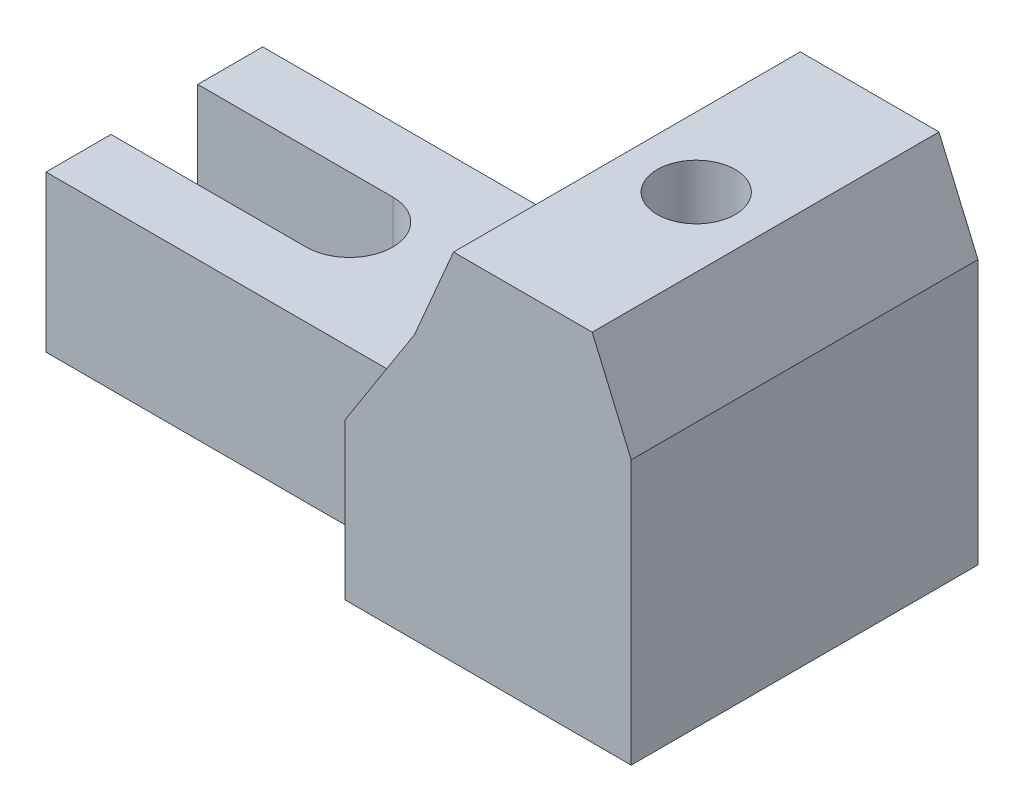
ISO-10303-21;
HEADER;
FILE_DESCRIPTION(('STEP AP214'),'2;1');
FILE_NAME('part.step','',(''),(''),'','','');
FILE_SCHEMA(('AUTOMOTIVE_DESIGN { 1 0 10303 214 1 1 1 1 }'));
ENDSEC;
DATA;
#1=APPLICATION_CONTEXT('core data for automotive mechanical design processes');
#2=APPLICATION_PROTOCOL_DEFINITION('international standard','automotive_design',2000,#1);
#3=PRODUCT_CONTEXT('',#1,'mechanical');
#4=PRODUCT('Part','Part','',(#3));
#5=PRODUCT_RELATED_PRODUCT_CATEGORY('part','',(#4));
#6=PRODUCT_DEFINITION_FORMATION('','',#4);
#7=PRODUCT_DEFINITION_CONTEXT('part definition',#1,'design');
#8=PRODUCT_DEFINITION('design','',#6,#7);
#9=PRODUCT_DEFINITION_SHAPE('','',#8);
#10=(LENGTH_UNIT() NAMED_UNIT(*) SI_UNIT(.MILLI.,.METRE.));
#11=(NAMED_UNIT(*) PLANE_ANGLE_UNIT() SI_UNIT($,.RADIAN.));
#12=(NAMED_UNIT(*) SI_UNIT($,.STERADIAN.) SOLID_ANGLE_UNIT());
#13=UNCERTAINTY_MEASURE_WITH_UNIT(LENGTH_MEASURE(1.E-05),#10,'distance_accuracy_value','');
#14=(GEOMETRIC_REPRESENTATION_CONTEXT(3) GLOBAL_UNCERTAINTY_ASSIGNED_CONTEXT((#13)) GLOBAL_UNIT_ASSIGNED_CONTEXT((#10,
#11,#12)) REPRESENTATION_CONTEXT('',''));
#15=CARTESIAN_POINT('',(0.,0.,0.));
#16=DIRECTION('',(0.,0.,1.));
#17=DIRECTION('',(1.,0.,0.));
#18=AXIS2_PLACEMENT_3D('',#15,#16,#17);
#19=CARTESIAN_POINT('',(0.,0.,80.));
#20=DIRECTION('',(1.,0.,0.));
#21=DIRECTION('',(0.,0.,-1.));
#22=AXIS2_PLACEMENT_3D('',#19,#20,#21);
#23=PLANE('',#22);
#24=DIRECTION('',(0.,-1.,0.));
#25=VECTOR('',#24,1.);
#26=CARTESIAN_POINT('',(0.,36.,15.));
#27=LINE('',#26,#25);
#28=CARTESIAN_POINT('',(0.,36.,15.));
#29=VERTEX_POINT('',#28);
#30=CARTESIAN_POINT('',(0.,0.,15.));
#31=VERTEX_POINT('',#30);
#32=EDGE_CURVE('E177',#29,#31,#27,.T.);
#33=ORIENTED_EDGE('',*,*,#32,.F.);
#34=DIRECTION('',(0.,0.,-1.));
#35=VECTOR('',#34,1.);
#36=CARTESIAN_POINT('',(0.,36.,80.));
#37=LINE('',#36,#35);
#38=CARTESIAN_POINT('',(0.,36.,0.));
#39=VERTEX_POINT('',#38);
#40=EDGE_CURVE('E93',#29,#39,#37,.T.);
#41=ORIENTED_EDGE('',*,*,#40,.T.);
#42=DIRECTION('',(0.,-1.,0.));
#43=VECTOR('',#42,1.);
#44=CARTESIAN_POINT('',(0.,0.,0.));
#45=LINE('',#44,#43);
#46=CARTESIAN_POINT('',(0.,0.,0.));
#47=VERTEX_POINT('',#46);
#48=EDGE_CURVE('E145',#39,#47,#45,.T.);
#49=ORIENTED_EDGE('',*,*,#48,.T.);
#50=DIRECTION('',(0.,0.,-1.));
#51=VECTOR('',#50,1.);
#52=CARTESIAN_POINT('',(0.,0.,80.));
#53=LINE('',#52,#51);
#54=EDGE_CURVE('E52',#31,#47,#53,.T.);
#55=ORIENTED_EDGE('',*,*,#54,.F.);
#56=EDGE_LOOP('',(#33,#41,#49,#55));
#57=FACE_BOUND('',#56,.T.);
#58=ADVANCED_FACE('F44',(#57),#23,.F.);
#59=CARTESIAN_POINT('',(0.,36.,80.));
#60=VERTEX_POINT('',#59);
#61=CARTESIAN_POINT('',(0.,36.,65.));
#62=VERTEX_POINT('',#61);
#63=EDGE_CURVE('E157',#60,#62,#37,.T.);
#64=ORIENTED_EDGE('',*,*,#63,.T.);
#65=DIRECTION('',(0.,-1.,0.));
#66=VECTOR('',#65,1.);
#67=CARTESIAN_POINT('',(0.,36.,65.));
#68=LINE('',#67,#66);
#69=CARTESIAN_POINT('',(0.,0.,65.));
#70=VERTEX_POINT('',#69);
#71=EDGE_CURVE('E186',#62,#70,#68,.T.);
#72=ORIENTED_EDGE('',*,*,#71,.T.);
#73=CARTESIAN_POINT('',(0.,0.,80.));
#74=VERTEX_POINT('',#73);
#75=EDGE_CURVE('E11',#74,#70,#53,.T.);
#76=ORIENTED_EDGE('',*,*,#75,.F.);
#77=DIRECTION('',(0.,-1.,0.));
#78=VECTOR('',#77,1.);
#79=CARTESIAN_POINT('',(0.,0.,80.));
#80=LINE('',#79,#78);
#81=EDGE_CURVE('E149',#60,#74,#80,.T.);
#82=ORIENTED_EDGE('',*,*,#81,.F.);
#83=EDGE_LOOP('',(#64,#72,#76,#82));
#84=FACE_BOUND('',#83,.T.);
#85=ADVANCED_FACE('F50',(#84),#23,.F.);
#86=CARTESIAN_POINT('',(0.,0.,80.));
#87=DIRECTION('',(0.,1.,0.));
#88=DIRECTION('',(0.,0.,1.));
#89=AXIS2_PLACEMENT_3D('',#86,#87,#88);
#90=PLANE('',#89);
#91=DIRECTION('',(1.,0.,0.));
#92=VECTOR('',#91,1.);
#93=CARTESIAN_POINT('',(0.,0.,0.));
#94=LINE('',#93,#92);
#95=CARTESIAN_POINT('',(66.,0.,0.));
#96=VERTEX_POINT('',#95);
#97=EDGE_CURVE('E154',#47,#96,#94,.T.);
#98=ORIENTED_EDGE('',*,*,#97,.T.);
#99=DIRECTION('',(0.,0.,-1.));
#100=VECTOR('',#99,1.);
#101=CARTESIAN_POINT('',(66.,0.,80.));
#102=LINE('',#101,#100);
#103=CARTESIAN_POINT('',(66.,0.,80.));
#104=VERTEX_POINT('',#103);
#105=EDGE_CURVE('E130',#104,#96,#102,.T.);
#106=ORIENTED_EDGE('',*,*,#105,.F.);
#107=DIRECTION('',(1.,0.,0.));
#108=VECTOR('',#107,1.);
#109=CARTESIAN_POINT('',(0.,0.,80.));
#110=LINE('',#109,#108);
#111=EDGE_CURVE('E97',#74,#104,#110,.T.);
#112=ORIENTED_EDGE('',*,*,#111,.F.);
#113=ORIENTED_EDGE('',*,*,#75,.T.);
#114=DIRECTION('',(-1.,0.,0.));
#115=VECTOR('',#114,1.);
#116=CARTESIAN_POINT('',(0.,0.,65.));
#117=LINE('',#116,#115);
#118=CARTESIAN_POINT('',(-84.,0.,65.));
#119=VERTEX_POINT('',#118);
#120=EDGE_CURVE('E58',#70,#119,#117,.T.);
#121=ORIENTED_EDGE('',*,*,#120,.T.);
#122=DIRECTION('',(0.,0.,-1.));
#123=VECTOR('',#122,1.);
#124=CARTESIAN_POINT('',(-84.,0.,65.));
#125=LINE('',#124,#123);
#126=CARTESIAN_POINT('',(-84.,0.,50.));
#127=VERTEX_POINT('',#126);
#128=EDGE_CURVE('E215',#119,#127,#125,.T.);
#129=ORIENTED_EDGE('',*,*,#128,.T.);
#130=DIRECTION('',(1.,0.,0.));
#131=VECTOR('',#130,1.);
#132=CARTESIAN_POINT('',(-39.,0.,50.));
#133=LINE('',#132,#131);
#134=CARTESIAN_POINT('',(-39.,0.,50.));
#135=VERTEX_POINT('',#134);
#136=EDGE_CURVE('E214',#127,#135,#133,.T.);
#137=ORIENTED_EDGE('',*,*,#136,.T.);
#138=CARTESIAN_POINT('',(-39.,0.,40.));
#139=DIRECTION('',(0.,1.,0.));
#140=DIRECTION('',(0.,0.,-1.));
#141=AXIS2_PLACEMENT_3D('',#138,#139,#140);
#142=CIRCLE('',#141,10.);
#143=CARTESIAN_POINT('',(-39.,0.,30.));
#144=VERTEX_POINT('',#143);
#145=EDGE_CURVE('E217',#135,#144,#142,.T.);
#146=ORIENTED_EDGE('',*,*,#145,.T.);
#147=DIRECTION('',(-1.,0.,0.));
#148=VECTOR('',#147,1.);
#149=CARTESIAN_POINT('',(-39.,0.,30.));
#150=LINE('',#149,#148);
#151=CARTESIAN_POINT('',(-84.,0.,30.));
#152=VERTEX_POINT('',#151);
#153=EDGE_CURVE('E222',#144,#152,#150,.T.);
#154=ORIENTED_EDGE('',*,*,#153,.T.);
#155=DIRECTION('',(0.,0.,-1.));
#156=VECTOR('',#155,1.);
#157=CARTESIAN_POINT('',(-84.,0.,15.));
#158=LINE('',#157,#156);
#159=CARTESIAN_POINT('',(-84.,0.,15.));
#160=VERTEX_POINT('',#159);
#161=EDGE_CURVE('E221',#152,#160,#158,.T.);
#162=ORIENTED_EDGE('',*,*,#161,.T.);
#163=DIRECTION('',(1.,0.,0.));
#164=VECTOR('',#163,1.);
#165=CARTESIAN_POINT('',(0.,0.,15.));
#166=LINE('',#165,#164);
#167=EDGE_CURVE('E166',#160,#31,#166,.T.);
#168=ORIENTED_EDGE('',*,*,#167,.T.);
#169=ORIENTED_EDGE('',*,*,#54,.T.);
#170=EDGE_LOOP('',(#98,#106,#112,#113,#121,#129,#137,#146,#154,#162,#168,#169));
#171=FACE_BOUND('',#170,.T.);
#172=ADVANCED_FACE('F164',(#171),#90,.F.);
#173=CARTESIAN_POINT('',(66.,0.,80.));
#174=DIRECTION('',(-1.,0.,0.));
#175=DIRECTION('',(0.,0.,1.));
#176=AXIS2_PLACEMENT_3D('',#173,#174,#175);
#177=PLANE('',#176);
#178=DIRECTION('',(0.,1.,0.));
#179=VECTOR('',#178,1.);
#180=CARTESIAN_POINT('',(66.,0.,0.));
#181=LINE('',#180,#179);
#182=CARTESIAN_POINT('',(66.,61.,0.));
#183=VERTEX_POINT('',#182);
#184=EDGE_CURVE('E124',#96,#183,#181,.T.);
#185=ORIENTED_EDGE('',*,*,#184,.T.);
#186=DIRECTION('',(0.,0.,-1.));
#187=VECTOR('',#186,1.);
#188=CARTESIAN_POINT('',(66.,61.,80.));
#189=LINE('',#188,#187);
#190=CARTESIAN_POINT('',(66.,61.,80.));
#191=VERTEX_POINT('',#190);
#192=EDGE_CURVE('E116',#191,#183,#189,.T.);
#193=ORIENTED_EDGE('',*,*,#192,.F.);
#194=DIRECTION('',(0.,1.,0.));
#195=VECTOR('',#194,1.);
#196=CARTESIAN_POINT('',(66.,0.,80.));
#197=LINE('',#196,#195);
#198=EDGE_CURVE('E110',#104,#191,#197,.T.);
#199=ORIENTED_EDGE('',*,*,#198,.F.);
#200=ORIENTED_EDGE('',*,*,#105,.T.);
#201=EDGE_LOOP('',(#185,#193,#199,#200));
#202=FACE_BOUND('',#201,.T.);
#203=ADVANCED_FACE('F118',(#202),#177,.F.);
#204=CARTESIAN_POINT('',(16.,61.,80.));
#205=DIRECTION('',(0.842271400661511,-0.539053696423367,0.));
#206=DIRECTION('',(0.539053696423367,0.842271400661511,0.));
#207=AXIS2_PLACEMENT_3D('',#204,#205,#206);
#208=PLANE('',#207);
#209=DIRECTION('',(-0.539053696423367,-0.842271400661511,0.));
#210=VECTOR('',#209,1.);
#211=CARTESIAN_POINT('',(16.,61.,0.));
#212=LINE('',#211,#210);
#213=CARTESIAN_POINT('',(16.,61.,0.));
#214=VERTEX_POINT('',#213);
#215=EDGE_CURVE('E151',#214,#39,#212,.T.);
#216=ORIENTED_EDGE('',*,*,#215,.T.);
#217=ORIENTED_EDGE('',*,*,#40,.F.);
#218=DIRECTION('',(0.,0.,1.));
#219=VECTOR('',#218,1.);
#220=CARTESIAN_POINT('',(0.,36.,65.));
#221=LINE('',#220,#219);
#222=EDGE_CURVE('E197',#29,#62,#221,.T.);
#223=ORIENTED_EDGE('',*,*,#222,.T.);
#224=ORIENTED_EDGE('',*,*,#63,.F.);
#225=DIRECTION('',(-0.539053696423367,-0.842271400661511,0.));
#226=VECTOR('',#225,1.);
#227=CARTESIAN_POINT('',(16.,61.,80.));
#228=LINE('',#227,#226);
#229=CARTESIAN_POINT('',(16.,61.,80.));
#230=VERTEX_POINT('',#229);
#231=EDGE_CURVE('E66',#230,#60,#228,.T.);
#232=ORIENTED_EDGE('',*,*,#231,.F.);
#233=DIRECTION('',(0.,0.,-1.));
#234=VECTOR('',#233,1.);
#235=CARTESIAN_POINT('',(16.,61.,80.));
#236=LINE('',#235,#234);
#237=EDGE_CURVE('E126',#230,#214,#236,.T.);
#238=ORIENTED_EDGE('',*,*,#237,.T.);
#239=EDGE_LOOP('',(#216,#217,#223,#224,#232,#238));
#240=FACE_BOUND('',#239,.T.);
#241=ADVANCED_FACE('F191',(#240),#208,.F.);
#242=CARTESIAN_POINT('',(0.,0.,80.));
#243=DIRECTION('',(0.,0.,1.));
#244=DIRECTION('',(1.,0.,0.));
#245=AXIS2_PLACEMENT_3D('',#242,#243,#244);
#246=PLANE('',#245);
#247=ORIENTED_EDGE('',*,*,#81,.T.);
#248=ORIENTED_EDGE('',*,*,#111,.T.);
#249=ORIENTED_EDGE('',*,*,#198,.T.);
#250=DIRECTION('',(-0.393919298579168,0.919145030018058,0.));
#251=VECTOR('',#250,1.);
#252=CARTESIAN_POINT('',(57.,82.,80.));
#253=LINE('',#252,#251);
#254=CARTESIAN_POINT('',(57.,82.,80.));
#255=VERTEX_POINT('',#254);
#256=EDGE_CURVE('E115',#191,#255,#253,.T.);
#257=ORIENTED_EDGE('',*,*,#256,.T.);
#258=DIRECTION('',(-1.,0.,0.));
#259=VECTOR('',#258,1.);
#260=CARTESIAN_POINT('',(41.,82.,80.));
#261=LINE('',#260,#259);
#262=CARTESIAN_POINT('',(25.,82.,80.));
#263=VERTEX_POINT('',#262);
#264=EDGE_CURVE('E131',#255,#263,#261,.T.);
#265=ORIENTED_EDGE('',*,*,#264,.T.);
#266=DIRECTION('',(-0.393919298579168,-0.919145030018058,0.));
#267=VECTOR('',#266,1.);
#268=CARTESIAN_POINT('',(25.,82.,80.));
#269=LINE('',#268,#267);
#270=EDGE_CURVE('E133',#263,#230,#269,.T.);
#271=ORIENTED_EDGE('',*,*,#270,.T.);
#272=ORIENTED_EDGE('',*,*,#231,.T.);
#273=EDGE_LOOP('',(#247,#248,#249,#257,#265,#271,#272));
#274=FACE_BOUND('',#273,.T.);
#275=ADVANCED_FACE('F108',(#274),#246,.T.);
#276=CARTESIAN_POINT('',(0.,0.,0.));
#277=DIRECTION('',(0.,0.,1.));
#278=DIRECTION('',(1.,0.,0.));
#279=AXIS2_PLACEMENT_3D('',#276,#277,#278);
#280=PLANE('',#279);
#281=ORIENTED_EDGE('',*,*,#48,.F.);
#282=ORIENTED_EDGE('',*,*,#215,.F.);
#283=DIRECTION('',(-0.393919298579168,-0.919145030018058,0.));
#284=VECTOR('',#283,1.);
#285=CARTESIAN_POINT('',(25.,82.,0.));
#286=LINE('',#285,#284);
#287=CARTESIAN_POINT('',(25.,82.,0.));
#288=VERTEX_POINT('',#287);
#289=EDGE_CURVE('E253',#288,#214,#286,.T.);
#290=ORIENTED_EDGE('',*,*,#289,.F.);
#291=DIRECTION('',(-1.,0.,0.));
#292=VECTOR('',#291,1.);
#293=CARTESIAN_POINT('',(41.,82.,0.));
#294=LINE('',#293,#292);
#295=CARTESIAN_POINT('',(57.,82.,0.));
#296=VERTEX_POINT('',#295);
#297=EDGE_CURVE('E140',#296,#288,#294,.T.);
#298=ORIENTED_EDGE('',*,*,#297,.F.);
#299=DIRECTION('',(-0.393919298579168,0.919145030018058,0.));
#300=VECTOR('',#299,1.);
#301=CARTESIAN_POINT('',(57.,82.,0.));
#302=LINE('',#301,#300);
#303=EDGE_CURVE('E146',#183,#296,#302,.T.);
#304=ORIENTED_EDGE('',*,*,#303,.F.);
#305=ORIENTED_EDGE('',*,*,#184,.F.);
#306=ORIENTED_EDGE('',*,*,#97,.F.);
#307=EDGE_LOOP('',(#281,#282,#290,#298,#304,#305,#306));
#308=FACE_BOUND('',#307,.T.);
#309=ADVANCED_FACE('F174',(#308),#280,.F.);
#310=CARTESIAN_POINT('',(41.,82.,0.));
#311=DIRECTION('',(0.,1.,0.));
#312=DIRECTION('',(0.,0.,1.));
#313=AXIS2_PLACEMENT_3D('',#310,#311,#312);
#314=PLANE('',#313);
#315=CARTESIAN_POINT('',(41.,82.,40.));
#316=DIRECTION('',(0.,1.,0.));
#317=DIRECTION('',(0.,0.,1.));
#318=AXIS2_PLACEMENT_3D('',#315,#316,#317);
#319=CIRCLE('',#318,9.);
#320=CARTESIAN_POINT('',(41.,82.,49.));
#321=VERTEX_POINT('',#320);
#322=EDGE_CURVE('E226',#321,#321,#319,.T.);
#323=ORIENTED_EDGE('',*,*,#322,.F.);
#324=EDGE_LOOP('',(#323));
#325=FACE_BOUND('',#324,.T.);
#326=ORIENTED_EDGE('',*,*,#264,.F.);
#327=DIRECTION('',(0.,0.,1.));
#328=VECTOR('',#327,1.);
#329=CARTESIAN_POINT('',(57.,82.,0.));
#330=LINE('',#329,#328);
#331=EDGE_CURVE('E135',#296,#255,#330,.T.);
#332=ORIENTED_EDGE('',*,*,#331,.F.);
#333=ORIENTED_EDGE('',*,*,#297,.T.);
#334=DIRECTION('',(0.,0.,1.));
#335=VECTOR('',#334,1.);
#336=CARTESIAN_POINT('',(25.,82.,0.));
#337=LINE('',#336,#335);
#338=EDGE_CURVE('E144',#288,#263,#337,.T.);
#339=ORIENTED_EDGE('',*,*,#338,.T.);
#340=EDGE_LOOP('',(#326,#332,#333,#339));
#341=FACE_BOUND('',#340,.T.);
#342=ADVANCED_FACE('F263',(#325,#341),#314,.T.);
#343=CARTESIAN_POINT('',(57.,82.,0.));
#344=DIRECTION('',(0.919145030018058,0.393919298579168,0.));
#345=DIRECTION('',(-0.393919298579168,0.919145030018058,0.));
#346=AXIS2_PLACEMENT_3D('',#343,#344,#345);
#347=PLANE('',#346);
#348=ORIENTED_EDGE('',*,*,#256,.F.);
#349=ORIENTED_EDGE('',*,*,#192,.T.);
#350=ORIENTED_EDGE('',*,*,#303,.T.);
#351=ORIENTED_EDGE('',*,*,#331,.T.);
#352=EDGE_LOOP('',(#348,#349,#350,#351));
#353=FACE_BOUND('',#352,.T.);
#354=ADVANCED_FACE('F132',(#353),#347,.T.);
#355=CARTESIAN_POINT('',(25.,82.,0.));
#356=DIRECTION('',(-0.919145030018058,0.393919298579168,0.));
#357=DIRECTION('',(-0.393919298579168,-0.919145030018058,0.));
#358=AXIS2_PLACEMENT_3D('',#355,#356,#357);
#359=PLANE('',#358);
#360=ORIENTED_EDGE('',*,*,#270,.F.);
#361=ORIENTED_EDGE('',*,*,#338,.F.);
#362=ORIENTED_EDGE('',*,*,#289,.T.);
#363=ORIENTED_EDGE('',*,*,#237,.F.);
#364=EDGE_LOOP('',(#360,#361,#362,#363));
#365=FACE_BOUND('',#364,.T.);
#366=ADVANCED_FACE('F264',(#365),#359,.T.);
#367=CARTESIAN_POINT('',(41.,2.,40.));
#368=DIRECTION('',(0.,1.,0.));
#369=DIRECTION('',(0.,0.,1.));
#370=AXIS2_PLACEMENT_3D('',#367,#368,#369);
#371=CYLINDRICAL_SURFACE('',#370,9.);
#372=CARTESIAN_POINT('',(41.,2.,40.));
#373=DIRECTION('',(0.,1.,0.));
#374=DIRECTION('',(0.,0.,1.));
#375=AXIS2_PLACEMENT_3D('',#372,#373,#374);
#376=CIRCLE('',#375,9.);
#377=CARTESIAN_POINT('',(41.,2.,49.));
#378=VERTEX_POINT('',#377);
#379=EDGE_CURVE('E136',#378,#378,#376,.T.);
#380=ORIENTED_EDGE('',*,*,#379,.F.);
#381=EDGE_LOOP('',(#380));
#382=FACE_BOUND('',#381,.T.);
#383=ORIENTED_EDGE('',*,*,#322,.T.);
#384=EDGE_LOOP('',(#383));
#385=FACE_BOUND('',#384,.T.);
#386=ADVANCED_FACE('F270',(#382,#385),#371,.F.);
#387=CARTESIAN_POINT('',(41.,2.,40.));
#388=DIRECTION('',(0.,1.,0.));
#389=DIRECTION('',(0.,0.,1.));
#390=AXIS2_PLACEMENT_3D('',#387,#388,#389);
#391=PLANE('',#390);
#392=ORIENTED_EDGE('',*,*,#379,.T.);
#393=EDGE_LOOP('',(#392));
#394=FACE_BOUND('',#393,.T.);
#395=ADVANCED_FACE('F273',(#394),#391,.T.);
#396=CARTESIAN_POINT('',(0.,36.,65.));
#397=DIRECTION('',(0.,0.,1.));
#398=DIRECTION('',(1.,0.,0.));
#399=AXIS2_PLACEMENT_3D('',#396,#397,#398);
#400=PLANE('',#399);
#401=ORIENTED_EDGE('',*,*,#120,.F.);
#402=ORIENTED_EDGE('',*,*,#71,.F.);
#403=DIRECTION('',(-1.,0.,0.));
#404=VECTOR('',#403,1.);
#405=CARTESIAN_POINT('',(0.,36.,65.));
#406=LINE('',#405,#404);
#407=CARTESIAN_POINT('',(-84.,36.,65.));
#408=VERTEX_POINT('',#407);
#409=EDGE_CURVE('E229',#62,#408,#406,.T.);
#410=ORIENTED_EDGE('',*,*,#409,.T.);
#411=DIRECTION('',(0.,-1.,0.));
#412=VECTOR('',#411,1.);
#413=CARTESIAN_POINT('',(-84.,36.,65.));
#414=LINE('',#413,#412);
#415=EDGE_CURVE('E203',#408,#119,#414,.T.);
#416=ORIENTED_EDGE('',*,*,#415,.T.);
#417=EDGE_LOOP('',(#401,#402,#410,#416));
#418=FACE_BOUND('',#417,.T.);
#419=ADVANCED_FACE('F335',(#418),#400,.T.);
#420=CARTESIAN_POINT('',(0.,36.,15.));
#421=DIRECTION('',(0.,0.,-1.));
#422=DIRECTION('',(-1.,0.,0.));
#423=AXIS2_PLACEMENT_3D('',#420,#421,#422);
#424=PLANE('',#423);
#425=ORIENTED_EDGE('',*,*,#167,.F.);
#426=DIRECTION('',(0.,-1.,0.));
#427=VECTOR('',#426,1.);
#428=CARTESIAN_POINT('',(-84.,36.,15.));
#429=LINE('',#428,#427);
#430=CARTESIAN_POINT('',(-84.,36.,15.));
#431=VERTEX_POINT('',#430);
#432=EDGE_CURVE('E232',#431,#160,#429,.T.);
#433=ORIENTED_EDGE('',*,*,#432,.F.);
#434=DIRECTION('',(1.,0.,0.));
#435=VECTOR('',#434,1.);
#436=CARTESIAN_POINT('',(0.,36.,15.));
#437=LINE('',#436,#435);
#438=EDGE_CURVE('E205',#431,#29,#437,.T.);
#439=ORIENTED_EDGE('',*,*,#438,.T.);
#440=ORIENTED_EDGE('',*,*,#32,.T.);
#441=EDGE_LOOP('',(#425,#433,#439,#440));
#442=FACE_BOUND('',#441,.T.);
#443=ADVANCED_FACE('F357',(#442),#424,.T.);
#444=CARTESIAN_POINT('',(-84.,36.,15.));
#445=DIRECTION('',(-1.,0.,0.));
#446=DIRECTION('',(0.,0.,1.));
#447=AXIS2_PLACEMENT_3D('',#444,#445,#446);
#448=PLANE('',#447);
#449=ORIENTED_EDGE('',*,*,#161,.F.);
#450=DIRECTION('',(0.,-1.,0.));
#451=VECTOR('',#450,1.);
#452=CARTESIAN_POINT('',(-84.,36.,30.));
#453=LINE('',#452,#451);
#454=CARTESIAN_POINT('',(-84.,36.,30.));
#455=VERTEX_POINT('',#454);
#456=EDGE_CURVE('E231',#455,#152,#453,.T.);
#457=ORIENTED_EDGE('',*,*,#456,.F.);
#458=DIRECTION('',(0.,0.,-1.));
#459=VECTOR('',#458,1.);
#460=CARTESIAN_POINT('',(-84.,36.,15.));
#461=LINE('',#460,#459);
#462=EDGE_CURVE('E210',#455,#431,#461,.T.);
#463=ORIENTED_EDGE('',*,*,#462,.T.);
#464=ORIENTED_EDGE('',*,*,#432,.T.);
#465=EDGE_LOOP('',(#449,#457,#463,#464));
#466=FACE_BOUND('',#465,.T.);
#467=ADVANCED_FACE('F370',(#466),#448,.T.);
#468=CARTESIAN_POINT('',(-39.,36.,30.));
#469=DIRECTION('',(0.,0.,1.));
#470=DIRECTION('',(1.,0.,0.));
#471=AXIS2_PLACEMENT_3D('',#468,#469,#470);
#472=PLANE('',#471);
#473=ORIENTED_EDGE('',*,*,#153,.F.);
#474=DIRECTION('',(0.,-1.,0.));
#475=VECTOR('',#474,1.);
#476=CARTESIAN_POINT('',(-39.,36.,30.));
#477=LINE('',#476,#475);
#478=CARTESIAN_POINT('',(-39.,36.,30.));
#479=VERTEX_POINT('',#478);
#480=EDGE_CURVE('E240',#479,#144,#477,.T.);
#481=ORIENTED_EDGE('',*,*,#480,.F.);
#482=DIRECTION('',(-1.,0.,0.));
#483=VECTOR('',#482,1.);
#484=CARTESIAN_POINT('',(-39.,36.,30.));
#485=LINE('',#484,#483);
#486=EDGE_CURVE('E505',#479,#455,#485,.T.);
#487=ORIENTED_EDGE('',*,*,#486,.T.);
#488=ORIENTED_EDGE('',*,*,#456,.T.);
#489=EDGE_LOOP('',(#473,#481,#487,#488));
#490=FACE_BOUND('',#489,.T.);
#491=ADVANCED_FACE('F377',(#490),#472,.T.);
#492=CARTESIAN_POINT('',(-39.,36.,40.));
#493=DIRECTION('',(0.,-1.,0.));
#494=DIRECTION('',(0.,0.,-1.));
#495=AXIS2_PLACEMENT_3D('',#492,#493,#494);
#496=CYLINDRICAL_SURFACE('',#495,10.);
#497=ORIENTED_EDGE('',*,*,#145,.F.);
#498=DIRECTION('',(0.,-1.,0.));
#499=VECTOR('',#498,1.);
#500=CARTESIAN_POINT('',(-39.,36.,50.));
#501=LINE('',#500,#499);
#502=CARTESIAN_POINT('',(-39.,36.,50.));
#503=VERTEX_POINT('',#502);
#504=EDGE_CURVE('E238',#503,#135,#501,.T.);
#505=ORIENTED_EDGE('',*,*,#504,.F.);
#506=CARTESIAN_POINT('',(-39.,36.,40.));
#507=DIRECTION('',(0.,1.,0.));
#508=DIRECTION('',(0.,0.,-1.));
#509=AXIS2_PLACEMENT_3D('',#506,#507,#508);
#510=CIRCLE('',#509,10.);
#511=EDGE_CURVE('E498',#503,#479,#510,.T.);
#512=ORIENTED_EDGE('',*,*,#511,.T.);
#513=ORIENTED_EDGE('',*,*,#480,.T.);
#514=EDGE_LOOP('',(#497,#505,#512,#513));
#515=FACE_BOUND('',#514,.T.);
#516=ADVANCED_FACE('F392',(#515),#496,.F.);
#517=CARTESIAN_POINT('',(-39.,36.,50.));
#518=DIRECTION('',(0.,0.,-1.));
#519=DIRECTION('',(-1.,0.,0.));
#520=AXIS2_PLACEMENT_3D('',#517,#518,#519);
#521=PLANE('',#520);
#522=ORIENTED_EDGE('',*,*,#136,.F.);
#523=DIRECTION('',(0.,-1.,0.));
#524=VECTOR('',#523,1.);
#525=CARTESIAN_POINT('',(-84.,36.,50.));
#526=LINE('',#525,#524);
#527=CARTESIAN_POINT('',(-84.,36.,50.));
#528=VERTEX_POINT('',#527);
#529=EDGE_CURVE('E204',#528,#127,#526,.T.);
#530=ORIENTED_EDGE('',*,*,#529,.F.);
#531=DIRECTION('',(1.,0.,0.));
#532=VECTOR('',#531,1.);
#533=CARTESIAN_POINT('',(-39.,36.,50.));
#534=LINE('',#533,#532);
#535=EDGE_CURVE('E494',#528,#503,#534,.T.);
#536=ORIENTED_EDGE('',*,*,#535,.T.);
#537=ORIENTED_EDGE('',*,*,#504,.T.);
#538=EDGE_LOOP('',(#522,#530,#536,#537));
#539=FACE_BOUND('',#538,.T.);
#540=ADVANCED_FACE('F401',(#539),#521,.T.);
#541=CARTESIAN_POINT('',(-84.,36.,65.));
#542=DIRECTION('',(-1.,0.,0.));
#543=DIRECTION('',(0.,0.,1.));
#544=AXIS2_PLACEMENT_3D('',#541,#542,#543);
#545=PLANE('',#544);
#546=ORIENTED_EDGE('',*,*,#128,.F.);
#547=ORIENTED_EDGE('',*,*,#415,.F.);
#548=DIRECTION('',(0.,0.,-1.));
#549=VECTOR('',#548,1.);
#550=CARTESIAN_POINT('',(-84.,36.,65.));
#551=LINE('',#550,#549);
#552=EDGE_CURVE('E492',#408,#528,#551,.T.);
#553=ORIENTED_EDGE('',*,*,#552,.T.);
#554=ORIENTED_EDGE('',*,*,#529,.T.);
#555=EDGE_LOOP('',(#546,#547,#553,#554));
#556=FACE_BOUND('',#555,.T.);
#557=ADVANCED_FACE('F413',(#556),#545,.T.);
#558=CARTESIAN_POINT('',(-39.,36.,40.));
#559=DIRECTION('',(0.,-1.,0.));
#560=DIRECTION('',(0.,0.,-1.));
#561=AXIS2_PLACEMENT_3D('',#558,#559,#560);
#562=PLANE('',#561);
#563=ORIENTED_EDGE('',*,*,#409,.F.);
#564=ORIENTED_EDGE('',*,*,#222,.F.);
#565=ORIENTED_EDGE('',*,*,#438,.F.);
#566=ORIENTED_EDGE('',*,*,#462,.F.);
#567=ORIENTED_EDGE('',*,*,#486,.F.);
#568=ORIENTED_EDGE('',*,*,#511,.F.);
#569=ORIENTED_EDGE('',*,*,#535,.F.);
#570=ORIENTED_EDGE('',*,*,#552,.F.);
#571=EDGE_LOOP('',(#563,#564,#565,#566,#567,#568,#569,#570));
#572=FACE_BOUND('',#571,.T.);
#573=ADVANCED_FACE('F430',(#572),#562,.F.);
#574=CLOSED_SHELL('',(#58,#85,#172,#203,#241,#275,#309,#342,#354,#366,#386,#395,#419,#443,#467,
#491,#516,#540,#557,#573));
#575=MANIFOLD_SOLID_BREP('B2',#574);
#576=ADVANCED_BREP_SHAPE_REPRESENTATION('',(#18,#575),#14);
#577=SHAPE_DEFINITION_REPRESENTATION(#9,#576);
ENDSEC;
END-ISO-10303-21;
